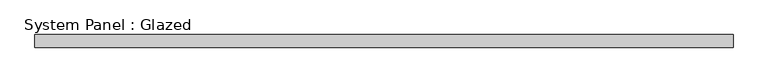
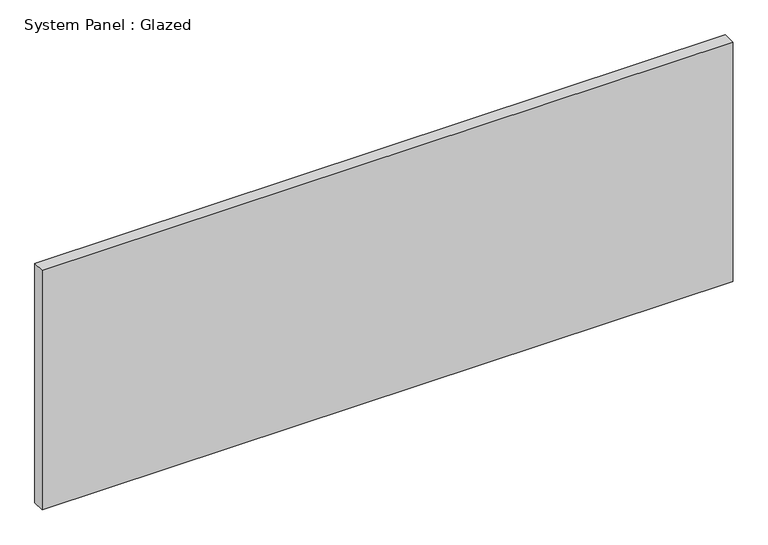
"""IFC4 building model written with IfcOpenShell, lengths in millimetres: plate geometry, System Panel : Glazed."""

from ifc_helpers import new_model, si_unit, origin, origin_with_axes, place, context, project, spatial, polyline, outline, extrude, source, transform, mapped, element, save


def system_panel_glazed_82e8a1e7(model_context):
    return source(origin(), model_context, "Body", "SweptSolid", [
        extrude(outline(polyline([(701.6749999, -44.45), (-701.6749999, -44.45), (-701.6749999, -19.05), (701.6749999, -19.05), (701.6749999, -44.45)])), origin_with_axes(), (0.0, 0.0, 1.0), 514.35),
    ])


if __name__ == "__main__":
    model = new_model("IFC4")
    model_context = context("Model", 3, world=origin())
    ifc_project = project(units=[si_unit("LENGTHUNIT", "METRE", prefix="MILLI")], contexts=[model_context])
    site = spatial("IfcSite", under=ifc_project)
    building = spatial("IfcBuilding", under=site)
    placement = place(None, origin())
    system_panel_glazed_shape = system_panel_glazed_82e8a1e7(model_context)
    element("IfcPlate", 1, ObjectType="System Panel : Glazed", at=placement, inside=building, context=model_context, shape_type="MappedRepresentation", body=[
        mapped(system_panel_glazed_shape, transform((0.0, 0.0, 0.0), x_axis=(1.0, 0.0, 0.0), y_axis=(0.0, 1.0, 0.0), z_axis=(0.0, 0.0, 1.0))),
    ])
    save(model, "model.ifc")

# Revit data of these elements
# Type "System Panel : Glazed"
#   Construction Type Id = "GSP4R"
#   Analytic Construction = "1/8 in Pilkington single glazing"
#   Visual Light Transmittance = 0.9
#   Solar Heat Gain Coefficient = 0.86
#   Heat Transfer Coefficient (U) = 1.18115 BTU/(h·ft²·°F)
#   Define Thermal Properties by = 1
# Element 1 (IfcPlate, "System Panel : Glazed")
#   Materials on its faces: "Glass"
# Materials
#   "Glass": class "Glass", colour RGB 0 128 192, transparency 0.75, Description = "Soda Lime Glass", Cost = 0
